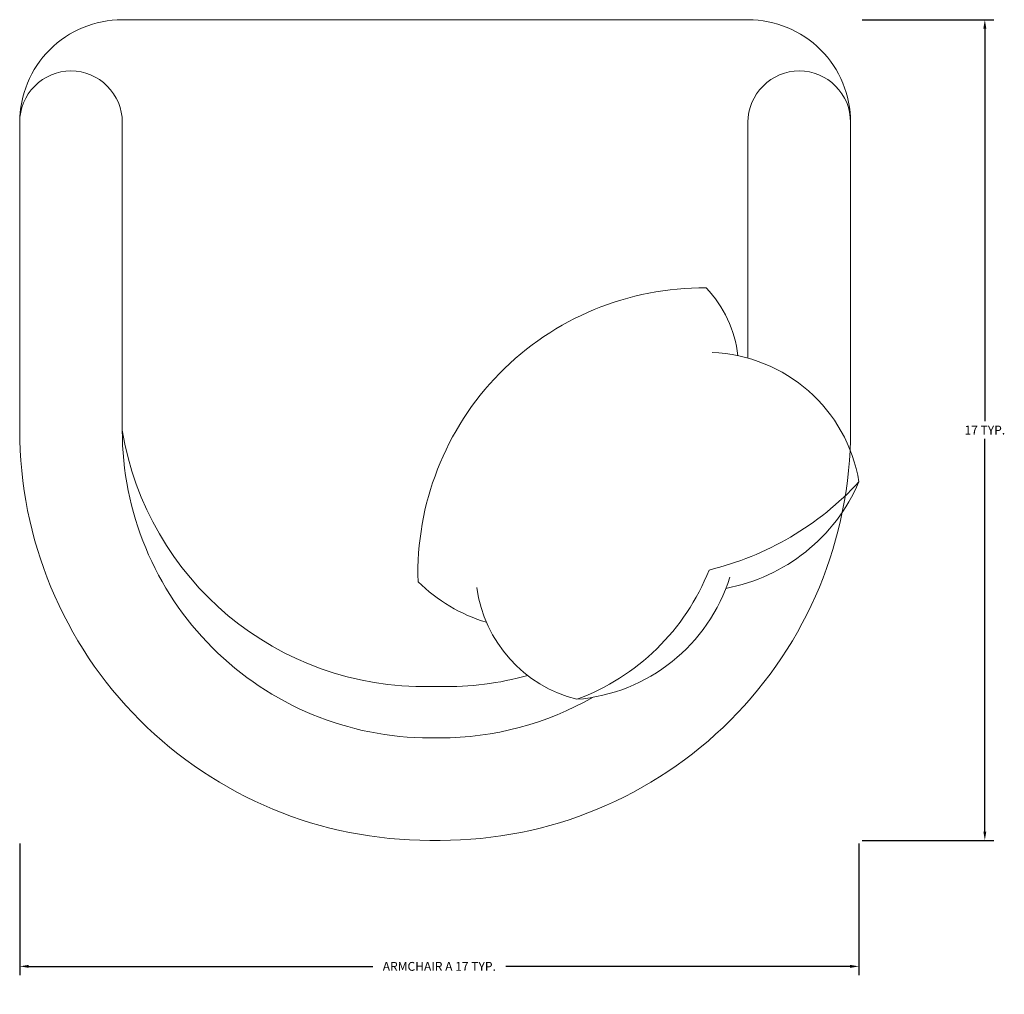
# Model space of a CAD drawing. Units: inches. Extents: x 963 to 2075, y 289 to 2657.
# Tile 71 of 98: x 1467.42 to 1487.48, y 2218.33 to 2238.18. Entities that reach past the tile are written whole.
import ezdxf

# ---------------------------------------------------------------- set-up
doc = ezdxf.new("R2010")
doc.units = ezdxf.units.IN
doc.layers.add('A-ANNO-DIMS', color=2, linetype='Continuous', lineweight=18)
doc.layers.add('A-FURN', color=8, linetype='Continuous', lineweight=18)
doc.styles.get("Standard").update_dxf_attribs({"font": 'arial.ttf'})
doc.dimstyles.get("Standard").update_dxf_attribs({"dimtxt": 0.18, "dimasz": 0.18, "dimexe": 0.18, "dimexo": 0.0625, "dimgap": 0.09, "dimtad": 0, "dimtih": 1, "dimtoh": 1, "dimdec": 4, "dimzin": 0, "dimdsep": 46, "dimtxsty": 'Standard', "dimcen": 0.09, "dimadec": 0, "dimazin": 0, "dimtfac": 1, "dimtdec": 4, "dimtofl": 0, "dimtmove": 0, "dimatfit": 3, "dimfxl": 1, "dimtolj": 1, "dimtzin": 0, "dimarcsym": 0})

# ---------------------------------------------------------------- blocks, each defined once
blk = doc.blocks.new('ARMCHAIR-A')
at = {"ltscale": 0.03}
blk.add_lwpolyline([(8.888, 17.178), (2.514, 17.178, 0.414214), (0.425, 15.088), (0.425, 8.819, 0.414214), (8.783, 0.461), (8.888, 0.461), (8.992, 0.461, 0.414214), (17.351, 8.819), (17.351, 15.088, 0.414214), (15.261, 17.178), (8.888, 17.178)], format="xyb", dxfattribs=at)
for points in [[(2.514, 8.819), (2.514, 15.088, 0.414214), (1.469, 16.133), (1.469, 16.133, 0.414214), (0.425, 15.088)], [(15.261, 10.284), (15.261, 15.088, -0.414214), (16.306, 16.133), (16.306, 16.133, -0.414214), (17.351, 15.088)], [(15.054, 10.334, 0.165541), (14.408, 11.715, 0.425989), (8.54, 5.729, 0.121523), (9.933, 4.904, -7.115464)], [(14.528, 10.398, -0.356772), (17.522, 7.764, -0.249542), (14.809, 5.594, 9.61688)], [(2.514, 8.819, 0.372719), (8.783, 3.595), (8.888, 3.595)], [(2.514, 8.819, 0.414214), (8.783, 2.55), (8.888, 2.55)], [(17.522, 7.764, -0.14773), (14.468, 5.969, -0.213343), (11.774, 3.335, -0.178662)], [(14.89, 5.826, -0.306663), (11.774, 3.335, -0.30633), (9.738, 5.61, 0.872847)], [(10.774, 3.82, -0.072384), (8.992, 3.595), (8.888, 3.595)], [(12.104, 3.377, -0.130591), (8.992, 2.55), (8.888, 2.55)]]:
    blk.add_lwpolyline(points, format="xyb")
blk = doc.blocks.new('*D22')
at = {"layer": 'A-ANNO-DIMS', "color": 0, "lineweight": -2, "transparency": 16777216}
for p, q in [((1467.425, 2221.398), (1467.425, 2218.716)), ((1484.522, 2221.398), (1484.522, 2218.716)), ((1467.605, 2218.896), (1474.616, 2218.896)), ((1484.342, 2218.896), (1477.331, 2218.896))]:
    blk.add_line(p, q, dxfattribs=at)
at = {"layer": 'A-ANNO-DIMS', "color": 0, "transparency": 16777216}
for points in [[(1467.605, 2218.926), (1467.605, 2218.866), (1467.425, 2218.896)], [(1484.342, 2218.926), (1484.342, 2218.866), (1484.522, 2218.896)]]:
    blk.add_solid(points, dxfattribs=at)
at = {"layer": 'Defpoints', "color": 0, "transparency": 16777216}
for p in [(1467.425, 2221.461), (1484.522, 2221.461), (1484.522, 2218.896)]:
    blk.add_point(p, dxfattribs=at)
at = {"layer": 'A-ANNO-DIMS', "color": 0, "transparency": 16777216, "insert": (1475.973, 2218.896), "char_height": 0.18, "attachment_point": 5}
blk.add_mtext('\\A1;ARMCHAIR A 17 TYP.', dxfattribs=at)
blk = doc.blocks.new('*D23')
at = {"layer": 'A-ANNO-DIMS', "color": 0, "lineweight": -2, "transparency": 16777216}
for p, q in [((1484.584, 2238.178), (1487.266, 2238.178)), ((1487.086, 2237.998), (1487.086, 2230)), ((1487.086, 2221.641), (1487.086, 2229.639)), ((1484.584, 2221.461), (1487.266, 2221.461))]:
    blk.add_line(p, q, dxfattribs=at)
at = {"layer": 'A-ANNO-DIMS', "color": 0, "transparency": 16777216}
for points in [[(1487.056, 2237.998), (1487.116, 2237.998), (1487.086, 2238.178)], [(1487.056, 2221.641), (1487.116, 2221.641), (1487.086, 2221.461)]]:
    blk.add_solid(points, dxfattribs=at)
at = {"layer": 'Defpoints', "color": 0, "transparency": 16777216}
for p in [(1484.522, 2238.178), (1487.086, 2238.178), (1484.522, 2221.461)]:
    blk.add_point(p, dxfattribs=at)
at = {"layer": 'A-ANNO-DIMS', "color": 0, "transparency": 16777216, "insert": (1487.086, 2229.819), "char_height": 0.18, "attachment_point": 5}
blk.add_mtext('\\A1;17 TYP.', dxfattribs=at)

msp = doc.modelspace()

# ---------------------------------------------------------------- block references
at = {"layer": 'A-FURN'}
msp.add_blockref('ARMCHAIR-A', (1467, 2221), dxfattribs=at)

# ---------------------------------------------------------------- dimensions: what is measured, and where the dimension line sits
at = {"layer": 'A-ANNO-DIMS'}
dim = msp.add_linear_dim(base=(1487.086, 2238.178), p1=(1484.522, 2221.461), p2=(1484.522, 2238.178), angle=90, text='<> TYP.', dimstyle='Standard', override={"dimdec": 0, "dimlfac": 1, "dimrnd": 0, "dimzin": 0, "dimdsep": 46, "dimlunit": 2}, dxfattribs=at)
dim.commit()
dim.dimension.update_dxf_attribs({"geometry": '*D23', "text_midpoint": (1487.086, 2229.819)})
dim = msp.add_linear_dim(base=(1484.522, 2218.896), p1=(1467.425, 2221.461), p2=(1484.522, 2221.461), text='ARMCHAIR A <> TYP.', dimstyle='Standard', override={"dimdec": 0, "dimlfac": 1, "dimrnd": 0, "dimzin": 0, "dimdsep": 46, "dimlunit": 2}, dxfattribs=at)
dim.commit()
dim.dimension.update_dxf_attribs({"geometry": '*D22', "text_midpoint": (1475.973, 2218.896)})

doc.saveas('drawing.dxf')
